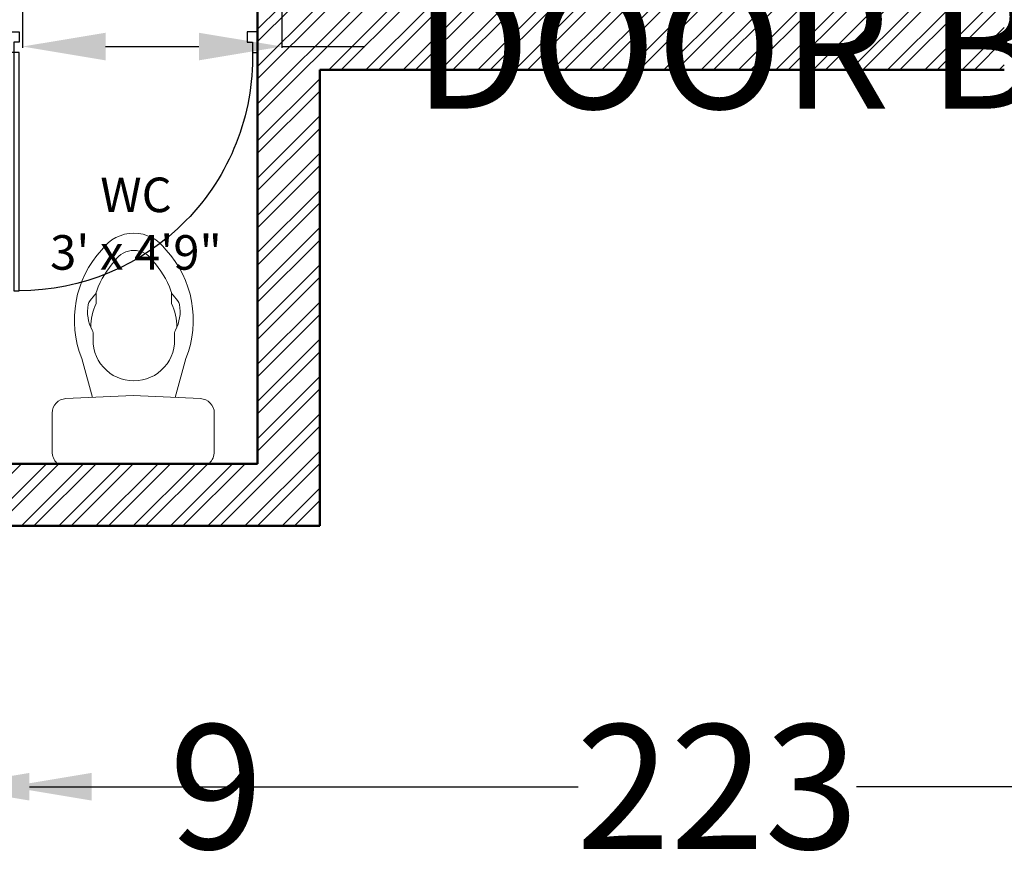
# Model space of a CAD drawing. Units: inches. Extents: x -90 to 536, y -553 to 299.
# Tile 2 of 27: x 49 to 191, y -553 to -430. Entities that reach past the tile are written whole.
import ezdxf

# ---------------------------------------------------------------- set-up
doc = ezdxf.new("R2010")
doc.units = ezdxf.units.IN
for name, color, linetype, lineweight in [('A-ANNO-DIMS', 2, 'Continuous', 18), ('A-AREA-IDEN', 7, 'Continuous', 18), ('A-DOOR', 4, 'Continuous', 25), ('A-FLOR-FIXT', 8, 'Continuous', 18), ('A-WALL-PATT', 252, 'Continuous', 13), ('Outer Wall', 1, 'Continuous', 50)]:
    doc.layers.add(name, color=color, linetype=linetype, lineweight=lineweight)
doc.styles.get("Standard").update_dxf_attribs({"font": 'arial.ttf'})
doc.dimstyles.get("Standard").update_dxf_attribs({"dimtxt": 18, "dimasz": 12, "dimexe": 0.18, "dimexo": 0.0625, "dimgap": 0.09, "dimtad": 0, "dimtih": 1, "dimtoh": 1, "dimdec": 0, "dimzin": 0, "dimdsep": 46, "dimlunit": 3, "dimtxsty": 'Standard', "dimcen": 0.09, "dimadec": 0, "dimazin": 0, "dimtfac": 1, "dimtdec": 0, "dimtofl": 0, "dimtmove": 0, "dimatfit": 3, "dimfxl": 1, "dimtolj": 1, "dimtzin": 0, "dimarcsym": 0})

# ---------------------------------------------------------------- blocks, each defined once
blk = doc.blocks.new('A$C1308471B')
at = {"ltscale": 20}
for p, q in [((0.0354, 0.4793), (0.1495, 0.4793)), ((0, 0.4607), (0, 0.0186)), ((0.2013, 0.2397), (0.1923, 0.4384)), ((0.1957, 0.3639), (0.3109, 0.3953)), ((0.5021, 0.3528), (0.4724, 0.3528)), ((0.4982, 0.3575), (0.4822, 0.3709)), ((0.2013, 0.2397), (0.1923, 0.0409)), ((0.1959, 0.1193), (0.3109, 0.0879)), ((0.5021, 0.1304), (0.4724, 0.1304)), ((0.4982, 0.1257), (0.4822, 0.1123)), ((0.0354, 0), (0.1495, 0))]:
    blk.add_line(p, q, dxfattribs=at)
for centre, radius, start, end in [((0.0354, 0.4328), 0.0465, 90, 136.5269), ((0.1495, 0.4365), 0.0429, 2.5755, 90), ((0.006, 0.4607), 0.006, 136.5269, 180), ((0.4248, 0.1104), 0.3068, 47.4135, 111.7924), ((0.4494, 0.2636), 0.1148, 79.3968, 118.5742), ((0.3654, 0.2416), 0.1206, 83.3523, 180), ((0.3823, 0.3868), 0.0255, 263.3523, 298.5742), ((0.405, 0.2159), 0.153, 63.502, 90.4522), ((0.4658, 0.3513), 0.0255, 50, 79.3968), ((0.5146, 0.377), 0.0255, 230, 251.3881), ((0.5021, 0.3273), 0.0255, 70.3751, 90), ((0.4248, 0.1104), 0.2558, 46.612, 70.3751), ((0.5654, 0.2416), 0.116, 0, 54.7115), ((0.5654, 0.2416), 0.065, 0, 57.2974), ((0.3654, 0.2416), 0.1206, 180, 276.6477), ((0.5654, 0.2416), 0.065, 302.7026, 0), ((0.5654, 0.2416), 0.116, 305.2885, 0), ((0.4248, 0.3728), 0.2558, 289.6249, 313.388), ((0.4248, 0.3728), 0.3068, 248.2076, 312.5865), ((0.3823, 0.0964), 0.0255, 61.4258, 96.6477), ((0.4494, 0.2196), 0.1148, 241.4258, 280.6032), ((0.405, 0.2673), 0.153, 269.5478, 296.498), ((0.5146, 0.1062), 0.0255, 108.6119, 130), ((0.5021, 0.1559), 0.0255, 270, 289.6249), ((0.4658, 0.1319), 0.0255, 280.6032, 310), ((0.1495, 0.0429), 0.0429, 270, 357.4245), ((0.006, 0.0186), 0.006, 180, 223.4731), ((0.0354, 0.0465), 0.0465, 223.4731, 270)]:
    blk.add_arc(centre, radius, start, end, dxfattribs=at)
blk = doc.blocks.new('DOOR-36-B')
for points in [[(37.5, 36), (37.5, 34.5), (36, 34.5), (36, 35.25), (34.5, 35.25), (34.5, 36)], [(0, 0.75), (0, 1.5), (34.5, 1.5), (34.5, 0.75)], [(37.5, 0), (37.5, 1.5), (36, 1.5), (36, 0.75), (34.5, 0.75), (34.5, 0)]]:
    blk.add_lwpolyline(points, close=True)
blk.add_arc((33.76, 1.5), 33.76, 88.7408, 180)
blk = doc.blocks.new('*D27')
at = {"layer": 'A-ANNO-DIMS', "color": 0, "lineweight": -2, "transparency": 16777216}
for p, q in [((49.13, -428.62), (49.13, -434.36)), ((86.63, -428.62), (86.63, -434.36)), ((61.13, -434.18), (74.63, -434.18)), ((86.63, -434.18), (98.63, -434.18))]:
    blk.add_line(p, q, dxfattribs=at)
at = {"layer": 'A-ANNO-DIMS', "color": 0, "transparency": 16777216}
for points in [[(61.13, -432.18), (61.13, -436.18), (49.13, -434.18)], [(74.63, -432.18), (74.63, -436.18), (86.63, -434.18)]]:
    blk.add_solid(points, dxfattribs=at)
at = {"layer": 'Defpoints', "color": 0, "transparency": 16777216}
for p in [(49.13, -428.55), (86.63, -428.55), (86.63, -434.18)]:
    blk.add_point(p, dxfattribs=at)
at = {"layer": 'A-ANNO-DIMS', "color": 0, "transparency": 16777216, "insert": (195.17, -434.18), "char_height": 18, "attachment_point": 5}
blk.add_mtext('\\A1;DOOR B 38 TYP.', dxfattribs=at)
blk = doc.blocks.new('*D51')
at = {"layer": 'A-ANNO-DIMS', "color": 0, "lineweight": -2, "transparency": 16777216}
for p, q in [((96.81, -393.34), (96.81, -404.61)), ((171.13, -393.34), (171.13, -404.61)), ((108.81, -404.43), (159.13, -404.43)), ((171.13, -404.43), (183.13, -404.43))]:
    blk.add_line(p, q, dxfattribs=at)
at = {"layer": 'A-ANNO-DIMS', "color": 0, "transparency": 16777216}
for points in [[(108.81, -402.43), (108.81, -406.43), (96.81, -404.43)], [(159.13, -402.43), (159.13, -406.43), (171.13, -404.43)]]:
    blk.add_solid(points, dxfattribs=at)
at = {"layer": 'Defpoints', "color": 0, "transparency": 16777216}
for p in [(96.81, -393.28), (171.13, -393.28), (171.13, -404.43)]:
    blk.add_point(p, dxfattribs=at)
at = {"layer": 'A-ANNO-DIMS', "color": 0, "transparency": 16777216, "insert": (274.99, -404.43), "char_height": 18, "attachment_point": 5}
blk.add_mtext('\\A1;SINGLE BED 74', dxfattribs=at)
blk = doc.blocks.new('*D54')
at = {"layer": 'A-ANNO-DIMS', "color": 0, "lineweight": -2, "transparency": 16777216}
for p, q in [((113.07, 249.45), (-2.85, 249.45)), ((-2.67, 237.45), (-2.67, -117.77)), ((-2.67, -491.55), (-2.67, -136.34)), ((38.07, -503.55), (-2.85, -503.55))]:
    blk.add_line(p, q, dxfattribs=at)
at = {"layer": 'A-ANNO-DIMS', "color": 0, "transparency": 16777216}
for points in [[(-4.67, 237.45), (-0.67, 237.45), (-2.67, 249.45)], [(-4.67, -491.55), (-0.67, -491.55), (-2.67, -503.55)]]:
    blk.add_solid(points, dxfattribs=at)
at = {"layer": 'Defpoints', "color": 0, "transparency": 16777216}
for p in [(-2.67, 249.45), (113.13, 249.45), (38.13, -503.55)]:
    blk.add_point(p, dxfattribs=at)
at = {"layer": 'A-ANNO-DIMS', "color": 0, "transparency": 16777216, "insert": (-2.67, -127.05), "char_height": 18, "attachment_point": 5}
blk.add_mtext('\\A1;753', dxfattribs=at)
blk = doc.blocks.new('*D57')
at = {"layer": 'A-ANNO-DIMS', "color": 0, "lineweight": -2, "transparency": 16777216}
for p, q in [((47.13, -494.62), (47.13, -541.49)), ((38.13, -503.62), (38.13, -541.49)), ((26.13, -541.31), (14.13, -541.31)), ((59.13, -541.31), (71.13, -541.31))]:
    blk.add_line(p, q, dxfattribs=at)
at = {"layer": 'A-ANNO-DIMS', "color": 0, "transparency": 16777216}
for points in [[(26.13, -539.31), (26.13, -543.31), (38.13, -541.31)], [(59.13, -539.31), (59.13, -543.31), (47.13, -541.31)]]:
    blk.add_solid(points, dxfattribs=at)
at = {"layer": 'Defpoints', "color": 0, "transparency": 16777216}
for p in [(47.13, -494.55), (38.13, -503.55), (47.13, -541.31)]:
    blk.add_point(p, dxfattribs=at)
at = {"layer": 'A-ANNO-DIMS', "color": 0, "transparency": 16777216, "insert": (77.14, -541.31), "char_height": 18, "attachment_point": 5}
blk.add_mtext('\\A1;9', dxfattribs=at)
blk = doc.blocks.new('*D67')
at = {"layer": 'A-ANNO-DIMS', "color": 0, "lineweight": -2, "transparency": 16777216}
for p, q in [((261.13, -437.62), (261.13, -541.49)), ((38.13, -503.62), (38.13, -541.49)), ((50.13, -541.31), (129.5, -541.31)), ((249.13, -541.31), (169.76, -541.31))]:
    blk.add_line(p, q, dxfattribs=at)
at = {"layer": 'A-ANNO-DIMS', "color": 0, "transparency": 16777216}
for points in [[(50.13, -539.31), (50.13, -543.31), (38.13, -541.31)], [(249.13, -539.31), (249.13, -543.31), (261.13, -541.31)]]:
    blk.add_solid(points, dxfattribs=at)
at = {"layer": 'Defpoints', "color": 0, "transparency": 16777216}
for p in [(261.13, -437.55), (38.13, -503.55), (261.13, -541.31)]:
    blk.add_point(p, dxfattribs=at)
at = {"layer": 'A-ANNO-DIMS', "color": 0, "transparency": 16777216, "insert": (149.63, -541.31), "char_height": 18, "attachment_point": 5}
blk.add_mtext('\\A1;223', dxfattribs=at)

msp = doc.modelspace()

# ---------------------------------------------------------------- hatches: boundary and pattern name
at = {"layer": 'A-WALL-PATT'}
h = msp.add_hatch(dxfattribs=at)
h.set_pattern_fill('ANSI32', color=256, scale=0.4)
h.set_pattern_definition([(45, (-88.8105, -603.6155), (-2.694077, 2.694077), []), (45, (-87.0145, -603.6155), (-2.694077, 2.694077), [])])
h.paths.add_polyline_path([(285.1317, 246.4462), (131.1317, 246.4462), (131.1317, 237.4462), (285.1317, 237.4462)])
h.paths.add_polyline_path([(122.1317, 237.4462), (113.1317, 237.4462), (113.1317, 152.4462), (122.1317, 152.4462), (122.1317, 166.4704)])
h.paths.add_polyline_path([(303.1317, 237.4462), (294.1317, 237.4462), (294.1317, 152.4462), (303.1317, 152.4462)])
h.paths.add_polyline_path([(47.1317, 91.9277), (38.1317, 91.9277), (38.1317, -6.5538), (77.1317, -6.5538), (77.1317, 2.4462), (70.5655, 2.4462), (47.1317, 2.4462)])
h.paths.add_polyline_path([(83.052, -61.5538), (47.1317, -61.5538), (47.1317, -24.5538), (38.1317, -24.5538), (38.1317, -70.5538), (74.052, -70.5538), (74.052, -223.5538), (38.1317, -223.5538), (38.1317, -503.5538), (92.1317, -503.5538), (92.1317, -437.5538), (191.1317, -437.5538), (191.1317, -428.5538), (83.1317, -428.5538), (83.1317, -494.5538), (47.1317, -494.5538), (47.1317, -232.5538), (83.052, -232.5538), (83.052, -70.5538)])
h.paths.add_polyline_path([(407.1317, -63.5538), (381.1317, -63.5538), (381.1317, 91.9277), (372.1317, 91.9277), (372.1317, 32.8805), (372.1317, -63.5538), (306.5745, -63.5538), (237.1317, -63.5538), (237.1317, -38.5538), (233.1317, -38.5538), (233.1317, -71.5538), (398.1317, -71.5538), (398.1317, -152.5538), (233.1317, -152.5538), (233.1317, -161.5538), (398.1317, -161.5538), (398.1317, -368.5538), (233.1317, -368.5538), (233.1317, -377.5538), (407.1317, -377.5538), (407.1317, -161.5538)])
h.paths.add_polyline_path([(261.1317, -422.5538), (252.1317, -422.5538), (252.1317, -428.5538), (233.1317, -428.5538), (233.1317, -437.5538), (261.1317, -437.5538)])
h.paths.add_polyline_path([(191.1317, -368.5538), (180.1317, -368.5538), (180.1317, -335.5538), (131.5919, -335.5538), (131.5919, -344.5538), (171.1317, -344.5538), (171.1317, -392.5538), (180.1317, -392.5538), (180.1317, -377.5538), (191.1317, -377.5538)], flags=17)
h.paths.add_polyline_path([(180.1317, -223.5538), (152.1317, -223.5538), (152.1317, -227.5538), (176.1317, -227.5538), (176.1317, -335.5538), (180.1317, -335.5538)], flags=17)
h.paths.add_polyline_path([(131.5919, -335.5538), (83.1317, -335.5538), (83.1317, -339.5538), (83.1317, -392.5538), (87.1317, -392.5538), (87.1317, -339.5538), (131.5919, -339.5538)], flags=17)
h.paths.add_polyline_path([(197.1317, 2.4462), (77.1317, 2.4462), (77.1317, -1.5538), (113.1317, -1.5538), (113.1317, -71.5538), (181.1317, -71.5538), (181.1317, -67.5538), (117.1317, -67.5538), (117.1317, -1.5538), (177.1317, -1.5538), (177.1317, -37.5538), (181.1317, -37.5538), (181.1317, -1.5538), (197.1317, -1.5538)])
h.paths.add_polyline_path([(173.1317, 138.4462), (122.1317, 138.4462), (122.1317, 134.4462), (173.1317, 134.4462)])
h.paths.add_polyline_path([(213.1317, 237.4462), (209.1317, 237.4462), (209.1317, 134.4462), (233.1317, 134.4462), (233.1317, 68.8889), (233.1317, -2.5538), (237.1317, -2.5538), (237.1317, 134.4462), (258.1317, 134.4462), (258.1317, 138.4462), (213.1317, 138.4462)])

# ---------------------------------------------------------------- linework, layer by layer
at = {"layer": 'Outer Wall'}
for p, q in [((83.1317, -428.5538), (83.1317, -494.5538)), ((191.1317, -437.5538), (92.1317, -437.5538)), ((92.1317, -437.5538), (92.1317, -503.5538)), ((83.1317, -494.5538), (47.1317, -494.5538)), ((92.1317, -503.5538), (38.1317, -503.5538))]:
    msp.add_line(p, q, dxfattribs=at)

# ---------------------------------------------------------------- block references
at = {"layer": 'A-DOOR', "extrusion": (0, 0, -1), "zscale": -1, "rotation": 89.99999999999979}
msp.add_blockref('DOOR-36-B', (-47.1317, -469.529), dxfattribs=at)
at = {"layer": 'A-FLOR-FIXT', "xscale": -48.95497407897215, "yscale": 48.95497407897215, "zscale": 48.95497407897215, "rotation": 270}
msp.add_blockref('A$C1308471B', (53.3985, -494.5538), dxfattribs=at)

# ---------------------------------------------------------------- texts
at = {"layer": 'A-AREA-IDEN', "insert": (90.2088, -453.143), "char_height": 5, "attachment_point": 3}
msp.add_mtext_dynamic_manual_height_columns('\\pxqc;{\\fTimes New Roman|b0|i0|c0|p18;WC\\P3\' x 4\'9"}', width=49.342153, gutter_width=12.5, heights=[0], dxfattribs=at)

# ---------------------------------------------------------------- dimensions: what is measured, and where the dimension line sits
at = {"layer": 'A-ANNO-DIMS'}
dim = msp.add_linear_dim(base=(-2.6677, 249.4462), p1=(38.1317, -503.5538), p2=(113.1317, 249.4462), angle=90, dimstyle='Standard', override={"dimdec": 0, "dimlfac": 1, "dimrnd": 0, "dimzin": 0, "dimdsep": 46, "dimlunit": 2}, dxfattribs=at)
dim.commit()
dim.dimension.update_dxf_attribs({"geometry": '*D54', "text_midpoint": (-2.6677, -127.0538)})
for base, p1, p2, text, picture, middle in [((171.1317, -404.4263), (96.8056, -393.2773), (171.1317, -393.2773), 'SINGLE BED <>', '*D51', (274.9898, -404.4263)), ((86.6317404714, -434.1787825705), (49.1317404714, -428.5537825705), (86.6317404714, -428.5537825705), 'DOOR B <> TYP.', '*D27', (195.1739914946, -434.1787825705))]:
    dim = msp.add_linear_dim(base=base, p1=p1, p2=p2, text=text, dimstyle='Standard', override={"dimdec": 0, "dimlfac": 1, "dimrnd": 0, "dimzin": 0, "dimdsep": 46, "dimlunit": 2}, dxfattribs=at)
    dim.commit()
    dim.dimension.update_dxf_attribs({"geometry": picture, "text_midpoint": middle})
for base, p2, picture, middle in [((261.1317, -541.3088), (261.1317, -437.5538), '*D67', (149.6317, -541.3088)), ((47.1317, -541.3088), (47.1317, -494.5538), '*D57', (77.1399, -541.3088))]:
    dim = msp.add_linear_dim(base=base, p1=(38.1317, -503.5538), p2=p2, dimstyle='Standard', override={"dimdec": 0, "dimlfac": 1, "dimrnd": 0, "dimzin": 0, "dimdsep": 46, "dimlunit": 2}, dxfattribs=at)
    dim.commit()
    dim.dimension.update_dxf_attribs({"geometry": picture, "text_midpoint": middle})

doc.saveas('drawing.dxf')
